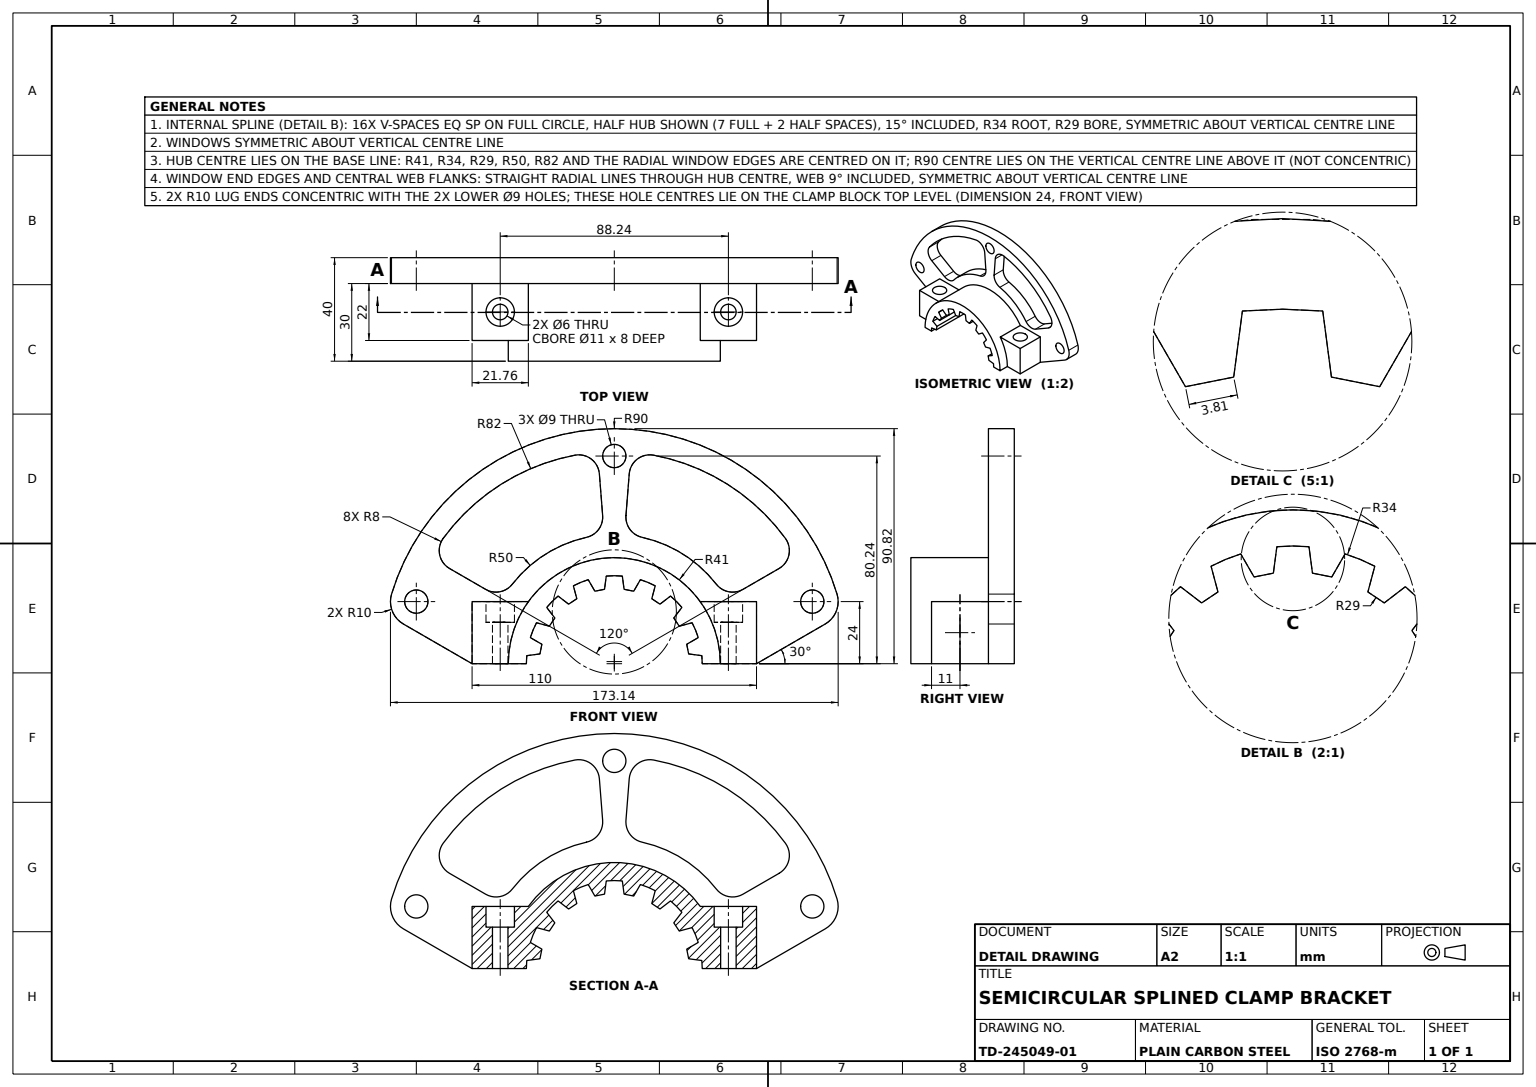
SolidWorks part; units mm, degrees
material "Plain Carbon Steel"
ref_plane "Front Plane" through (0, 0, 0) normal (0, 0, 1) x (1, 0, 0)
ref_plane "Top Plane" through (0, 0, 0) normal (0, 1, 0) x (1, 0, 0)
ref_plane "Right Plane" through (0, 0, 0) normal (1, 0, 0) x (0, 0, -1)
sketch "Sector Plate Sketch" plane through (0, 0, 0) normal (0, 0, 1) x (1, 0, 0)
  line L0 (0, 0) -> (55, 0)
  line L1 (55, 0) -> (81.5692, 15.3397)
  line L2 (0, 0) -> (-55, 0)
  line L3 (-55, 0) -> (-81.5692, 15.3397)
  line L4 (0, 0) -> (0, -41.9579) construction
  line L5 (0, 0) -> (0, 100.4174) construction
  line L6 (4.5071, 57.2685) -> (5.7719, 73.3395)
  line L7 (-4.5071, 57.2685) -> (-5.7719, 73.3395)
  line L8 (49.7494, 28.7228) -> (63.7103, 36.7831)
  line L9 (-49.7494, 28.7228) -> (-63.7103, 36.7831)
  line L10 (-3.923, 49.8459) -> (0, 0) construction
  arc A3 (-86.1404, 26.8971) -> (86.1404, 26.8971) centre (0, 0.8234) cw
  arc A4 (81.5692, 15.3397) -> (86.1404, 26.8971) centre (76.5692, 24) ccw
  arc A5 (-81.5692, 15.3397) -> (-86.1404, 26.8971) centre (-76.5692, 24) cw
  circle A6 centre (-76.5692, 24) radius 4.5
  circle A7 centre (76.5692, 24) radius 4.5
  arc A8 (-76.5692, 24) -> (76.5692, 24) centre (0, 0) cw construction
  circle A9 centre (0, 80.2424) radius 4.5
  arc A10 (-39.4391, 30.7336) -> (-10.7608, 48.8283) centre (0, 0) cw
  arc A11 (66.1654, 48.4369) -> (15.2335, 80.5726) centre (0, 0) ccw
  arc A12 (-15.2335, 80.5726) -> (-66.1654, 48.4369) centre (0, 0) ccw
  arc A13 (10.7608, 48.8283) -> (39.4391, 30.7336) centre (0, 0) cw
  arc A14 (63.7103, 36.7831) -> (66.1654, 48.4369) centre (59.7103, 43.7114) ccw
  arc A15 (39.4391, 30.7336) -> (49.7494, 28.7228) centre (45.7494, 35.651) ccw
  arc A16 (4.5071, 57.2685) -> (10.7608, 48.8283) centre (12.4825, 56.6409) ccw
  arc A17 (5.7719, 73.3395) -> (15.2335, 80.5726) centre (13.7473, 72.7118) cw
  arc A18 (-4.5071, 57.2685) -> (-10.7608, 48.8283) centre (-12.4825, 56.6409) cw
  arc A19 (-5.7719, 73.3395) -> (-15.2335, 80.5726) centre (-13.7473, 72.7118) ccw
  arc A20 (-66.1654, 48.4369) -> (-63.7103, 36.7831) centre (-59.7103, 43.7114) ccw
  arc A21 (-39.4391, 30.7336) -> (-49.7494, 28.7228) centre (-45.7494, 35.651) cw
  point P9 (88.1202, 19.1219)
  point P13 (-88.1202, 19.1219)
  point P29 (71.0141, 41)
  point P32 (43.3013, 25)
  point P35 (3.923, 49.8459)
  point P43 (-6.4336, 81.7472)
  point P46 (-71.0141, 41)
  point P49 (-43.3013, 25)
  dimension "D2" = 90
  dimension "D3" = 10
  dimension "D6" = 9
  dimension "D8" = 50
  dimension "D9" = 32
  dimension "D10" = 8
  dimension "D1" = 120
  dimension "D4" = 110
  dimension "D5" = 24
  dimension "D7" = 9
extrude "Sector Plate" add sketch "Sector Plate Sketch" along normal blind 10
sketch "Mounting Lug Sketch" plane through (0, 0, 10) normal (0, 0, 1) x (1, 0, 0)
  line L1 (-55, 0) -> (55, 0)
  line L2 (-55, 0) -> (-55, 24)
  line L3 (-55, 24) -> (55, 24)
  line L4 (55, 0) -> (55, 24)
  dimension "D1" = 24
extrude "Mounting Lugs" add sketch "Mounting Lug Sketch" along normal blind 22
sketch "Half Hub Sketch" plane through (0, 0, 10) normal (0, 0, 1) x (1, 0, 0)
  line L0 (-55, 0) -> (55, 0) construction
  line L1 (-41, 0) -> (41, 0)
  arc A0 (-41, 0) -> (41, 0) centre (0, 0) cw
  dimension "D1" = 41
extrude "Half Hub" add sketch "Half Hub Sketch" along normal blind 30
hole_wizard "Lug C'Bore Holes Ø6" positions "3DSketch1" profile "Sketch5" legacy
sketch3d "3DSketch1"
  line L0 (-33.2415, 24, 32) -> (-55, 24, 32) construction
  line L1 (55, 24, 32) -> (33.2415, 24, 32) construction
  line L2 (-55, 24, 21) -> (55, 24, 21) construction
  line L3 (-55, 24, 32) -> (-55, 24, 10) construction
  line L4 (55, 24, 32) -> (55, 24, 10) construction
  point P0 (-44.1208, 24, 21)
  point P2 (44.1208, 24, 21)
  point P7 (-44.1208, 24, 32)
  point P11 (44.1208, 24, 32)
sketch "Sketch5" plane through (-44.1208, 24, 21) normal (1, 0, 0) x (0, 0, 1)
  line L0 (0, 0) -> (0, 99.9687)
  line L1 (0, 99.9687) -> (3, 99.9687)
  line L2 (3, 99.9687) -> (3, 8)
  line L3 (3, 8) -> (5.5, 8)
  line L4 (5.5, 8) -> (5.5, 0)
  line L5 (5.5, 0) -> (0, 0)
  line L6 (0, 110) -> (0, -10) construction
  dimension "Diameter" = 6
  dimension "Depth" = 100
  dimension "C-Bore Diameter" = 11
  dimension "C-Bore Depth" = 8
sketch "Internal Spline Sketch" plane through (0, 0, 40) normal (0, 0, 1) x (1, 0, 0)
  line L0 (-41, 0) -> (41, 0) construction
  line L1 (0, 0) -> (0, 50.065) construction
  line L2 (-3.1073, 33.8577) -> (-3.7794, 28.7527)
  line L3 (3.1073, 33.8577) -> (3.7794, 28.7527)
  line L4 (-3.7794, 28.7527) -> (-7.9354, -2.8155) construction
  line L5 (3.7794, 28.7527) -> (8.0229, -3.4805) construction
  line L6 (10.086, 32.4695) -> (7.5115, 28.0103)
  line L7 (15.8275, 30.0914) -> (14.4948, 25.1177)
  line L8 (21.7439, 26.1382) -> (17.6588, 23.0036)
  line L9 (26.1382, 21.7439) -> (23.0036, 17.6588)
  line L10 (30.0914, 15.8275) -> (25.1177, 14.4948)
  line L11 (32.4695, 10.086) -> (28.0103, 7.5115)
  line L12 (33.8577, 3.1073) -> (28.7527, 3.7794)
  line L13 (-33.8577, 3.1073) -> (-28.7527, 3.7794)
  line L14 (0, 0) -> (24.0416, 24.0416) construction
  line L15 (-34, 0) -> (34, 0)
  line L16 (-32.4695, 10.086) -> (-28.0103, 7.5115)
  line L17 (33.8577, -3.1073) -> (28.7527, -3.7794) [skipped]
  line L18 (-30.0914, 15.8275) -> (-25.1177, 14.4948)
  line L19 (-26.1382, 21.7439) -> (-23.0036, 17.6588)
  line L20 (-21.7439, 26.1382) -> (-17.6588, 23.0036)
  line L21 (-15.8275, 30.0914) -> (-14.4948, 25.1177)
  line L22 (-10.086, 32.4695) -> (-7.5115, 28.0103)
  arc A0 (-3.1073, 33.8577) -> (3.1073, 33.8577) centre (0, 0) cw
  arc A1 (-28.7527, 3.7794) -> (-28.0103, 7.5115) centre (0, 0) cw
  circle A2 centre (0, 0) radius 7.5 construction
  arc A3 (3.7794, 28.7527) -> (7.5115, 28.0103) centre (0, 0) cw
  arc A4 (10.086, 32.4695) -> (15.8275, 30.0914) centre (0, 0) cw
  arc A5 (21.7439, 26.1382) -> (26.1382, 21.7439) centre (0, 0) cw
  arc A6 (30.0914, 15.8275) -> (32.4695, 10.086) centre (0, 0) cw
  arc A7 (33.8577, 3.1073) -> (34, 0) centre (0, 0) cw
  arc A8 (14.4948, 25.1177) -> (17.6588, 23.0036) centre (0, 0) cw
  arc A9 (23.0036, 17.6588) -> (25.1177, 14.4948) centre (0, 0) cw
  arc A10 (28.0103, 7.5115) -> (28.7527, 3.7794) centre (0, 0) cw
  arc A11 (-33.8577, 3.1073) -> (-34, 0) centre (0, 0) ccw
  arc A12 (-28.0103, 7.5115) -> (-28.7527, 3.7794) centre (0, 0) ccw
  arc A13 (-30.0914, 15.8275) -> (-32.4695, 10.086) centre (0, 0) ccw
  arc A14 (-21.7439, 26.1382) -> (-26.1382, 21.7439) centre (0, 0) ccw
  arc A15 (-10.086, 32.4695) -> (-15.8275, 30.0914) centre (0, 0) ccw
  arc A16 (-25.1177, 14.4948) -> (-23.0036, 17.6588) centre (0, 0) cw
  arc A17 (-17.6588, 23.0036) -> (-14.4948, 25.1177) centre (0, 0) cw
  arc A18 (-7.5115, 28.0103) -> (-3.7794, 28.7527) centre (0, 0) cw
  line M17 (-41, 0) -> (41, 0)
  dimension "D1" = 34
  dimension "D2" = 29
  dimension "D4" = 15
  dimension "D3" = 15
  dimension "D6" = 45
  dimension "D5" = 5
extrude "Internal Spline Cut" cut sketch "Internal Spline Sketch" against normal through all contours A18 L22 A15 L21 A17 L20 A14 L19 A16 L18 A13 L16 A1 L13 A11 A7 L12 A10 L11 A6 L10 A9 L9 A5 L8 A8 L7 A4 L6 A3 L3 A0 L2 M17
